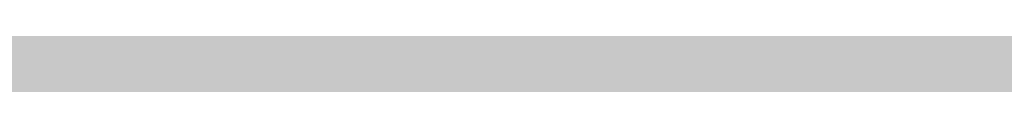
# Model space of a CAD drawing. Units: feet. Extents: x 3168 to 4724, y 827 to 1477.
# Tile 69 of 256: x 3273.17306 to 3273.20669, y 1099.01485 to 1099.01628. Entities that reach past the tile are written whole.
import ezdxf

# ---------------------------------------------------------------- set-up
doc = ezdxf.new("R2010")
doc.units = ezdxf.units.FT
doc.layers.add('A-ELEV', color=7, linetype='Continuous', lineweight=35)
doc.layers.add('A-ELEV-PATT', color=8, linetype='Continuous', lineweight=13)

msp = doc.modelspace()

# ---------------------------------------------------------------- hatches: boundary and pattern name
at = {"layer": 'A-ELEV-PATT'}
h = msp.add_hatch(color=256, dxfattribs=at)
h.dxf.hatch_style = 1
edge = h.paths.add_edge_path()
edge.add_ellipse((3552.905762, 979.220141), major_axis=(36.744924, 0), ratio=0.484848485, start_angle=0, end_angle=360)
edge = h.paths.add_edge_path()
edge.add_ellipse((3559.891637, 929.252282), major_axis=(36.744924, 0), ratio=0.484848485, start_angle=0, end_angle=360)
edge = h.paths.add_edge_path()
edge.add_line((3299.31681, 1198.606081), (3479.916714, 1198.606081))
edge.add_line((3479.916714, 1198.606081), (3479.916714, 1209.86857))
edge.add_spline(control_points=[(3479.916714, 1209.86857), (3464.301157, 1209.86857), (3448.685601, 1209.86857), (3410.949139, 1209.86857), (3388.828234, 1209.86857), (3355.646876, 1209.86857), (3344.586423, 1209.86857), (3327.995745, 1209.86857), (3322.465518, 1209.86857), (3314.170179, 1209.86857), (3311.405066, 1209.86857), (3307.257396, 1209.86857), (3305.874839, 1209.86857), (3303.801005, 1209.86857), (3303.109726, 1209.86857), (3302.072809, 1209.86857), (3301.72717, 1209.86857), (3301.208711, 1209.86857), (3301.035891, 1209.86857), (3300.776662, 1209.86857), (3300.690252, 1209.86857), (3300.560638, 1209.86857), (3300.517433, 1209.86857), (3300.452625, 1209.86857), (3300.431023, 1209.86857), (3300.398619, 1209.86857), (3300.387818, 1209.86857), (3300.366216, 1209.86857), (3300.345676, 1209.86857), (3300.345548, 1209.86857), (3300.345505, 1209.86857), (3300.343304, 1209.86857), (3300.341146, 1209.868571), (3300.337909, 1209.868571), (3300.33683, 1209.868572), (3300.333942, 1209.868573), (3300.332133, 1209.868574), (3300.325515, 1209.868577), (3300.320706, 1209.868581), (3300.310925, 1209.868592), (3300.305952, 1209.868598), (3300.290511, 1209.868623), (3300.280045, 1209.868646), (3300.232425, 1209.868777), (3300.195298, 1209.868954), (3299.951068, 1209.870608), (3299.744824, 1209.874326), (3299.436827, 1209.883257), (3299.334389, 1209.886792), (3299.181079, 1209.89292), (3299.130033, 1209.895099), (3298.652217, 1209.916801), (3298.22946, 1209.945718), (3297.601631, 1210.002367), (3297.393404, 1210.023464), (3297.082652, 1210.058309), (3296.979332, 1210.070458), (3296.292954, 1210.154861), (3295.718148, 1210.243356), (3294.868717, 1210.39885), (3294.5877, 1210.454478), (3294.169341, 1210.543349), (3294.030415, 1210.573878), (3291.707149, 1211.1012), (3289.65359, 1211.813435), (3285.776259, 1213.563988), (3283.95141, 1214.603478), (3280.512159, 1216.98008), (3278.897241, 1218.317592), (3276.379914, 1220.829489), (3275.416042, 1221.917738), (3274.039342, 1223.7077), (3273.581043, 1224.349535), (3273.143228, 1225.016316)], knot_values=[39.119033, 39.119033, 39.119033, 39.119033, 39.286353, 39.286353, 39.523379, 39.523379, 39.641892, 39.641892, 39.701148, 39.701148, 39.730777, 39.730777, 39.745591, 39.745591, 39.752998, 39.752998, 39.756701, 39.756701, 39.758553, 39.758553, 39.759479, 39.759479, 39.759942, 39.759942, 39.760173, 39.760173, 39.760289, 39.760289, 39.760405, 39.760405, 39.760463, 39.760463, 39.763389, 39.763389, 39.764851, 39.764851, 39.767304, 39.767304, 39.773825, 39.773825, 39.78057, 39.78057, 39.79477, 39.79477, 39.845194, 39.845194, 40.126715, 40.126715, 40.267476, 40.267476, 40.337856, 40.337856, 40.927023, 40.927023, 41.221606, 41.221606, 41.368898, 41.368898, 42.202622, 42.202622, 42.619485, 42.619485, 42.827916, 42.827916, 46.118323, 46.118323, 49.408731, 49.408731, 52.699139, 52.699139, 54.927489, 54.927489, 56.104228, 56.104228, 56.104228, 56.104228], weights=[1, 1, 1, 1, 1, 1, 1, 1, 1, 1, 1, 1, 1, 1, 1, 1, 1, 1, 1, 1, 1, 1, 1, 1, 1, 1, 1, 1, 1, 1, 1, 1, 1, 1, 1, 1, 1, 1, 1, 1, 1, 1, 1, 1, 1, 1, 1, 1, 1, 1, 1, 1, 1, 1, 1, 1, 1, 1, 1, 1, 1, 1, 1, 1, 1, 1, 1, 1, 1, 1, 1, 1, 1, 1], degree=3, periodic=0)
edge.add_line((3273.143228, 1225.016316), (3273.143228, 1099.016316))
edge.add_line((3273.143228, 1099.016316), (3299.31681, 1099.016316))
edge.add_line((3299.31681, 1099.016316), (3299.31681, 1198.606081))
edge = h.paths.add_edge_path()
edge.add_line((3304.758443, 1324.15806), (3479.916714, 1324.15806))
edge.add_line((3479.916714, 1324.15806), (3479.916714, 1335.714618))
edge.add_line((3479.916714, 1335.714618), (3269.161628, 1335.714618))
edge.add_spline(control_points=[(3269.161628, 1335.714618), (3264.024231, 1335.714618), (3258.364118, 1328.958189), (3259.264311, 1323.900274)], knot_values=[0, 0, 0, 0, 15.412191, 15.412191, 15.412191, 15.412191], degree=3, periodic=0)
edge.add_line((3259.264311, 1323.900274), (3265.516849, 1288.769135))
edge.add_line((3265.516849, 1288.769135), (3275.265103, 1261.545626))
edge.add_line((3275.265103, 1261.545626), (3304.758443, 1261.545626))
edge.add_line((3304.758443, 1261.545626), (3304.758443, 1324.15806))
h = msp.add_hatch(color=256, dxfattribs=at)
h.dxf.hatch_style = 1
h.paths.add_polyline_path([(3384.525247, 1099.016316), (3335.029168, 1099.016316), (3299.31681, 1099.016316), (3273.143228, 1099.016316), (3217.565364, 1099.016316), (3168.069285, 827.11626), (3335.029168, 827.11626)])

# ---------------------------------------------------------------- linework, layer by layer
at = {"layer": 'A-ELEV'}
msp.add_open_spline([(3808.5202, 1099.016316), (3808.5202, 1141.413235), (3808.5202, 1183.810154), (3808.5202, 1226.635324), (3808.5202, 1227.063576), (3808.5202, 1227.491828), (3811.491871, 1248.994673), (3814.463542, 1270.497518), (3817.46523, 1292.217564), (3817.495247, 1292.434764), (3817.525264, 1292.651964), (3817.572801, 1310.106748), (3817.620339, 1327.561532), (3817.667877, 1345.016316), (3817.667877, 1345.457962), (3817.667877, 1345.899608), (3817.667877, 1346.456047), (3817.667877, 1346.57084), (3817.667877, 1346.752887), (3817.667877, 1346.820142), (3817.667877, 1346.93487), (3817.667877, 1346.982345), (3817.667877, 1347.038587), (3817.667877, 1347.047356), (3817.667877, 1347.073661), (3817.667877, 1347.059303), (3817.667877, 1347.061545), (3817.667876, 1347.062667), (3817.667875, 1347.066031), (3817.667874, 1347.068274), (3817.66787, 1347.075001), (3817.667866, 1347.079486), (3817.667849, 1347.092937), (3817.667833, 1347.101902), (3817.667766, 1347.12879), (3817.667699, 1347.146705), (3817.667432, 1347.200421), (3817.667165, 1347.236192), (3817.6661, 1347.343385), (3817.665038, 1347.414686), (3817.660812, 1347.628095), (3817.656608, 1347.769708), (3817.63997, 1348.192487), (3817.623509, 1348.471586), (3817.559094, 1349.300067), (3817.496121, 1349.840588), (3817.255432, 1351.424156), (3817.026318, 1352.428785), (3816.306871, 1354.888914), (3815.743745, 1356.268727), (3814.463959, 1358.81921), (3813.746413, 1359.990968), (3812.195838, 1362.172343), (3811.362245, 1363.182124), (3809.588836, 1365.069009), (3808.648816, 1365.946105), (3806.654262, 1367.579616), (3805.599702, 1368.336154), (3803.352891, 1369.722327), (3802.160535, 1370.352386), (3799.600813, 1371.453586), (3798.232688, 1371.925481), (3795.280084, 1372.634624), (3793.693148, 1372.872068), (3791.869441, 1372.92648), (3791.740861, 1372.92922), (3791.353371, 1372.934101), (3791.092707, 1372.932901), (3790.304116, 1372.915068), (3789.769543, 1372.884195), (3789.20919, 1372.830236), (3789.190622, 1372.828424), (3789.134892, 1372.822912), (3789.097705, 1372.819137), (3789.048445, 1372.814008), (3789.0364, 1372.812743), (3789.000256, 1372.808918), (3788.976147, 1372.806325), (3788.949405, 1372.803404), (3788.946786, 1372.803118), (3788.942567, 1372.802655), (3788.940967, 1372.80248), (3788.938572, 1372.802217), (3788.937777, 1372.802129), (3788.935391, 1372.801867), (3788.867535, 1372.794402), (3788.756866, 1372.782228), (3788.701532, 1372.776141), (3788.53553, 1372.75788), (3788.424861, 1372.745707), (3788.092856, 1372.709185), (3787.871519, 1372.684837), (3787.207509, 1372.611793), (3786.764835, 1372.563097), (3785.436814, 1372.417009), (3784.551467, 1372.319617), (3781.895425, 1372.027442), (3780.12473, 1371.832658), (3774.812646, 1371.248307), (3771.271256, 1370.858739), (3760.647088, 1369.690037), (3753.56431, 1368.910902), (3732.315973, 1366.573498), (3718.150416, 1365.015228), (3694.006758, 1362.359326), (3684.028657, 1361.261694), (3674.050557, 1360.164062), (3664.600662, 1360.164062), (3655.150767, 1360.164062), (3626.801081, 1360.164062), (3607.901291, 1360.164062), (3551.20192, 1360.164062), (3513.40234, 1360.164062), (3467.725182, 1360.164062), (3459.847604, 1360.164062), (3436.214873, 1360.164062), (3420.459718, 1360.164062), (3373.194255, 1360.164062), (3341.683946, 1360.164062), (3302.848162, 1360.164062), (3295.522686, 1360.164062), (3286.038292, 1360.164062), (3283.879372, 1360.164062), (3277.402613, 1360.164062), (3273.084773, 1360.164062), (3267.732851, 1360.164062), (3266.698768, 1360.164062), (3263.59652, 1360.164062), (3261.528355, 1360.164062), (3259.236943, 1360.164062), (3259.013697, 1360.164062), (3258.343958, 1360.164062), (3257.897466, 1360.164062), (3257.430998, 1360.164062), (3257.411022, 1360.164062), (3257.370573, 1360.164062), (3257.37547, 1360.164062), (3257.374598, 1360.164062), (3257.373937, 1360.164062), (3257.371956, 1360.164062), (3257.370635, 1360.164061), (3257.366673, 1360.16406), (3257.364032, 1360.164059), (3257.356109, 1360.164053), (3257.350828, 1360.164047), (3257.334987, 1360.164023), (3257.32443, 1360.163998), (3257.292769, 1360.163899), (3257.271676, 1360.163799), (3257.208439, 1360.163398), (3257.166337, 1360.162995), (3257.040206, 1360.161388), (3256.956349, 1360.159783), (3256.705504, 1360.153393), (3256.53924, 1360.147036), (3256.04357, 1360.121916), (3255.717296, 1360.097102), (3254.752446, 1360.000481), (3254.127968, 1359.906513), (3252.180067, 1359.525332), (3250.941574, 1359.143991), (3248.670175, 1358.24329), (3247.635739, 1357.723834), (3245.732632, 1356.603471), (3244.863388, 1356.00206), (3243.253108, 1354.742865), (3242.511972, 1354.084731), (3240.751052, 1352.344781), (3239.800961, 1351.229574), (3238.087769, 1348.87244), (3237.324685, 1347.630355), (3235.98251, 1344.971632), (3235.402205, 1343.554907), (3234.591081, 1340.815458), (3234.310882, 1339.54355), (3233.97649, 1336.802561), (3233.922113, 1335.330877), (3234.148916, 1332.591269), (3234.349529, 1331.367201), (3234.719893, 1329.999367), (3234.752423, 1329.883362), (3234.853619, 1329.534797), (3234.925892, 1329.301685), (3235.024836, 1329.002552), (3235.046924, 1328.936928), (3235.077639, 1328.847239), (3235.085924, 1328.823198), (3235.110939, 1328.751064), (3235.127828, 1328.702962), (3235.147992, 1328.646242), (3235.151059, 1328.637632), (3235.156096, 1328.623526), (3235.158061, 1328.61803), (3235.160209, 1328.61203), (3235.165612, 1328.596943), (3235.180099, 1328.556486), (3235.190263, 1328.528101), (3235.220756, 1328.442946), (3235.241084, 1328.386176), (3235.302069, 1328.215865), (3235.342726, 1328.102325), (3235.464696, 1327.761704), (3235.54601, 1327.534623), (3235.78995, 1326.853381), (3235.952577, 1326.39922), (3236.440459, 1325.036736), (3236.765713, 1324.128414), (3237.741475, 1321.403446), (3238.391983, 1319.586801), (3240.343508, 1314.136866), (3241.644525, 1310.503576), (3245.547574, 1299.603706), (3248.149607, 1292.337126), (3255.955706, 1270.537385), (3261.159772, 1256.004225), (3267.387618, 1238.612001), (3268.411397, 1235.752937), (3269.510378, 1232.683864), (3269.585579, 1232.473854), (3269.706612, 1232.135851), (3269.752444, 1232.007857), (3269.827329, 1231.79873), (3269.856382, 1231.717595), (3269.906325, 1231.578122), (3269.927215, 1231.519782), (3269.972468, 1231.393406), (3269.996831, 1231.325368), (3270.026503, 1231.242506), (3270.031811, 1231.227681), (3270.040282, 1231.204024), (3270.039224, 1231.206979), (3270.039359, 1231.206601), (3270.039427, 1231.206412), (3270.03963, 1231.205846), (3270.039765, 1231.205468), (3270.040171, 1231.204335), (3270.040442, 1231.203579), (3270.041254, 1231.201313), (3270.041796, 1231.199802), (3270.04342, 1231.195269), (3270.044504, 1231.192248), (3270.047756, 1231.183185), (3270.049926, 1231.177145), (3270.056442, 1231.159028), (3270.060793, 1231.146957), (3270.073867, 1231.110761), (3270.082613, 1231.086656), (3270.108936, 1231.014413), (3270.1266, 1230.96635), (3270.179934, 1230.822457), (3270.215947, 1230.726923), (3270.325323, 1230.441508), (3270.400026, 1230.252811), (3270.629249, 1229.691444), (3270.788883, 1229.323501), (3271.286488, 1228.238319), (3271.6431, 1227.539755), (3272.775859, 1225.515277), (3273.614169, 1224.260502), (3275.416042, 1221.917738), (3276.379914, 1220.829489), (3278.897241, 1218.317592), (3280.512159, 1216.98008), (3283.95141, 1214.603478), (3285.776259, 1213.563988), (3289.65359, 1211.813435), (3291.707149, 1211.1012), (3294.030415, 1210.573878), (3294.169341, 1210.543349), (3294.5877, 1210.454478), (3294.868717, 1210.39885), (3295.718148, 1210.243356), (3296.292954, 1210.154861), (3296.979332, 1210.070458), (3297.082652, 1210.058309), (3297.393404, 1210.023464), (3297.601631, 1210.002367), (3298.22946, 1209.945718), (3298.652217, 1209.916801), (3299.130033, 1209.895099), (3299.181079, 1209.89292), (3299.334389, 1209.886792), (3299.436827, 1209.883257), (3299.744824, 1209.874326), (3299.951068, 1209.870608), (3300.195298, 1209.868954), (3300.232425, 1209.868777), (3300.280045, 1209.868646), (3300.290511, 1209.868623), (3300.305952, 1209.868598), (3300.310925, 1209.868592), (3300.320706, 1209.868581), (3300.325515, 1209.868577), (3300.332133, 1209.868574), (3300.333942, 1209.868573), (3300.33683, 1209.868572), (3300.337909, 1209.868571), (3300.341146, 1209.868571), (3300.343304, 1209.86857), (3300.345505, 1209.86857), (3300.345548, 1209.86857), (3300.345676, 1209.86857), (3300.366216, 1209.86857), (3300.387818, 1209.86857), (3300.398619, 1209.86857), (3300.431023, 1209.86857), (3300.452625, 1209.86857), (3300.517433, 1209.86857), (3300.560638, 1209.86857), (3300.690252, 1209.86857), (3300.776662, 1209.86857), (3301.035891, 1209.86857), (3301.208711, 1209.86857), (3301.72717, 1209.86857), (3302.072809, 1209.86857), (3303.109726, 1209.86857), (3303.801005, 1209.86857), (3305.874839, 1209.86857), (3307.257396, 1209.86857), (3311.405066, 1209.86857), (3314.170179, 1209.86857), (3322.465518, 1209.86857), (3327.995745, 1209.86857), (3344.586423, 1209.86857), (3355.646876, 1209.86857), (3388.828234, 1209.86857), (3410.949139, 1209.86857), (3477.311855, 1209.86857), (3521.553665, 1209.86857), (3566.836184, 1209.86857), (3567.876892, 1209.86857), (3570.999017, 1209.86857), (3573.080433, 1209.86857), (3575.781396, 1209.86857), (3576.400943, 1209.86857), (3577.295821, 1209.86857), (3577.571152, 1209.86857), (3578.397146, 1209.86857), (3578.947808, 1209.86857), (3579.756491, 1209.86857), (3580.014511, 1209.86857), (3580.342737, 1209.86857), (3580.326865, 1209.86857), (3580.32717, 1209.86857), (3580.327323, 1209.86857), (3580.327781, 1209.86857), (3580.328086, 1209.86857), (3580.329002, 1209.86857), (3580.329613, 1209.86857), (3580.331445, 1209.86857), (3580.332667, 1209.86857), (3580.336332, 1209.868569), (3580.338775, 1209.868567), (3580.346107, 1209.868563), (3580.350995, 1209.868558), (3580.365663, 1209.86854), (3580.375445, 1209.868522), (3580.404801, 1209.868449), (3580.424386, 1209.868376), (3580.483183, 1209.868085), (3580.522437, 1209.867793), (3580.640361, 1209.866624), (3580.719195, 1209.865454), (3580.956315, 1209.860766), (3581.115222, 1209.85607), (3581.594164, 1209.83723), (3581.916419, 1209.818331), (3582.889947, 1209.742428), (3583.547986, 1209.666169), (3585.531827, 1209.360617), (3586.867216, 1209.053886), (3589.471545, 1208.252472), (3590.740241, 1207.757852), (3591.995451, 1207.158802), (3592.057809, 1207.12874), (3592.244242, 1207.037954), (3592.367676, 1206.976632), (3592.73528, 1206.790359), (3592.976752, 1206.663101), (3593.244539, 1206.516441), (3593.274731, 1206.499825), (3593.365115, 1206.449839), (3593.425113, 1206.416333), (3593.604314, 1206.315285), (3593.722725, 1206.247211), (3593.857212, 1206.168398), (3593.874362, 1206.158319), (3593.925741, 1206.128041), (3593.959899, 1206.107798), (3594.062086, 1206.046899), (3594.129827, 1206.006074), (3594.208436, 1205.958171), (3594.219683, 1205.951304), (3594.253391, 1205.930686), (3594.275819, 1205.916917), (3594.342972, 1205.875536), (3594.387563, 1205.847853), (3594.433616, 1205.81905), (3594.435256, 1205.818024), (3594.440175, 1205.814946), (3594.443453, 1205.812894), (3594.447123, 1205.810594), (3594.447516, 1205.810348), (3594.448695, 1205.80961), (3594.449481, 1205.809117), (3594.450366, 1205.808562), (3594.450466, 1205.8085), (3594.4506, 1205.808415), (3594.467399, 1205.797887), (3594.493269, 1205.781674), (3594.506204, 1205.773568), (3594.545008, 1205.749248), (3594.570878, 1205.733035), (3594.648487, 1205.684396), (3594.700226, 1205.651969), (3594.855444, 1205.554691), (3594.958922, 1205.489839), (3595.269357, 1205.295282), (3595.476314, 1205.165577), (3596.097185, 1204.776463), (3596.511099, 1204.517054), (3597.752841, 1203.738826), (3598.580669, 1203.220007), (3601.064152, 1201.663551), (3602.719807, 1200.625914), (3607.686774, 1197.513002), (3610.998085, 1195.437727), (3620.932018, 1189.211903), (3627.55464, 1185.061354), (3647.422507, 1172.609707), (3660.667751, 1164.308608), (3700.403484, 1139.405313), (3726.893973, 1122.803116), (3757.205715, 1103.806052), (3761.02697, 1101.411184), (3764.848224, 1099.016316), (3745.328271, 1099.016316), (3725.808319, 1099.016316), (3706.288366, 1099.016316), (3706.288366, 1108.453237), (3706.288366, 1117.890158), (3706.288366, 1127.327079), (3710.750754, 1127.327079), (3715.213143, 1127.327079), (3719.675531, 1127.327079)], degree=3, knots=[0, 0, 0, 0, 0.982037, 0.982037, 0.991957, 0.991957, 0.991957, 1.966522, 1.966522, 1.976367, 1.976367, 1.976367, 2.976367, 2.976367, 2.976367, 3.00169, 3.00169, 3.008272, 3.008272, 3.012129, 3.012129, 3.014851, 3.014851, 3.015353, 3.015353, 3.016359, 3.016359, 3.017365, 3.017365, 3.019376, 3.019376, 3.023398, 3.023398, 3.031442, 3.031442, 3.047531, 3.047531, 3.079708, 3.079708, 3.144063, 3.144063, 3.272772, 3.272772, 3.53019, 3.53019, 4.045026, 4.045026, 5.074698, 5.074698, 6.700878, 6.700878, 8.327058, 8.327058, 9.953238, 9.953238, 11.579418, 11.579418, 13.205598, 13.205598, 14.831778, 14.831778, 16.457958, 16.457958, 18.084138, 18.084138, 18.206872, 18.206872, 18.45234, 18.45234, 18.943275, 18.943275, 18.960093, 18.960093, 18.993729, 18.993729, 19.00461, 19.00461, 19.026374, 19.026374, 19.028737, 19.028737, 19.03018, 19.03018, 19.030897, 19.030897, 19.032332, 19.032332, 19.033766, 19.033766, 19.036636, 19.036636, 19.042374, 19.042374, 19.053851, 19.053851, 19.076805, 19.076805, 19.122714, 19.122714, 19.21453, 19.21453, 19.398163, 19.398163, 19.765429, 19.765429, 20.024128, 20.024128, 20.024128, 20.092031, 20.092031, 20.227836, 20.227836, 20.499446, 20.499446, 20.556051, 20.556051, 20.66926, 20.66926, 20.895678, 20.895678, 20.948316, 20.948316, 20.963829, 20.963829, 20.994855, 20.994855, 21.002285, 21.002285, 21.017146, 21.017146, 21.01875, 21.01875, 21.021959, 21.021959, 21.022102, 21.022102, 21.022249, 21.022249, 21.022708, 21.022708, 21.023627, 21.023627, 21.025464, 21.025464, 21.029138, 21.029138, 21.036486, 21.036486, 21.051183, 21.051183, 21.080575, 21.080575, 21.139361, 21.139361, 21.256932, 21.256932, 21.492073, 21.492073, 21.962356, 21.962356, 23.01002, 23.01002, 24.057684, 24.057684, 25.105348, 25.105348, 26.153011, 26.153011, 27.776787, 27.776787, 29.400562, 29.400562, 31.024337, 31.024337, 32.278801, 32.278801, 33.533265, 33.533265, 34.467568, 34.467568, 34.553971, 34.553971, 34.726776, 34.726776, 34.775309, 34.775309, 34.793079, 34.793079, 34.82862, 34.82862, 34.834979, 34.834979, 34.839039, 34.839039, 34.839411, 34.839411, 34.840285, 34.840285, 34.842034, 34.842034, 34.845531, 34.845531, 34.852525, 34.852525, 34.866512, 34.866512, 34.894488, 34.894488, 34.950439, 34.950439, 35.062342, 35.062342, 35.286147, 35.286147, 35.733758, 35.733758, 35.821815, 35.821815, 35.828283, 35.828283, 35.832225, 35.832225, 35.834724, 35.834724, 35.836521, 35.836521, 35.838617, 35.838617, 35.839073, 35.839073, 35.839345, 35.839345, 35.839617, 35.839617, 35.840161, 35.840161, 35.841249, 35.841249, 35.843425, 35.843425, 35.847778, 35.847778, 35.856482, 35.856482, 35.873891, 35.873891, 35.908709, 35.908709, 35.978345, 35.978345, 36.117617, 36.117617, 36.396161, 36.396161, 36.953248, 36.953248, 38.067423, 38.067423, 40.295772, 40.295772, 42.524122, 42.524122, 45.81453, 45.81453, 49.104937, 49.104937, 52.395345, 52.395345, 52.603776, 52.603776, 53.020639, 53.020639, 53.854363, 53.854363, 54.001655, 54.001655, 54.296238, 54.296238, 54.885405, 54.885405, 54.955785, 54.955785, 55.096546, 55.096546, 55.378067, 55.378067, 55.42849, 55.42849, 55.442691, 55.442691, 55.449436, 55.449436, 55.455957, 55.455957, 55.458409, 55.458409, 55.459872, 55.459872, 55.462798, 55.462798, 55.462856, 55.462856, 55.462972, 55.462972, 55.463088, 55.463088, 55.463319, 55.463319, 55.463782, 55.463782, 55.464708, 55.464708, 55.46656, 55.46656, 55.470263, 55.470263, 55.47767, 55.47767, 55.492484, 55.492484, 55.522112, 55.522112, 55.581369, 55.581369, 55.699882, 55.699882, 55.936907, 55.936907, 56.410959, 56.410959, 56.42211, 56.42211, 56.444413, 56.444413, 56.451051, 56.451051, 56.454001, 56.454001, 56.459901, 56.459901, 56.462666, 56.462666, 56.463418, 56.463418, 56.464171, 56.464171, 56.465675, 56.465675, 56.468684, 56.468684, 56.474702, 56.474702, 56.486738, 56.486738, 56.51081, 56.51081, 56.558955, 56.558955, 56.655243, 56.655243, 56.847821, 56.847821, 57.232975, 57.232975, 58.003284, 58.003284, 59.543901, 59.543901, 62.625137, 62.625137, 68.787607, 68.787607, 74.950078, 74.950078, 75.27336, 75.27336, 75.919923, 75.919923, 77.213051, 77.213051, 77.377769, 77.377769, 77.707206, 77.707206, 78.366079, 78.366079, 78.462532, 78.462532, 78.655436, 78.655436, 79.041245, 79.041245, 79.105735, 79.105735, 79.234714, 79.234714, 79.492672, 79.492672, 79.502197, 79.502197, 79.521249, 79.521249, 79.523534, 79.523534, 79.528103, 79.528103, 79.528682, 79.528682, 79.528885, 79.528885, 79.529089, 79.529089, 79.529495, 79.529495, 79.530308, 79.530308, 79.531935, 79.531935, 79.535187, 79.535187, 79.541693, 79.541693, 79.554704, 79.554704, 79.580725, 79.580725, 79.632769, 79.632769, 79.736856, 79.736856, 79.94503, 79.94503, 80.361377, 80.361377, 80.421435, 80.421435, 80.421435, 81.421435, 81.421435, 81.421435, 82.421435, 82.421435, 82.421435, 83.421435, 83.421435, 83.421435, 83.421435], dxfattribs=at)

doc.saveas('drawing.dxf')
